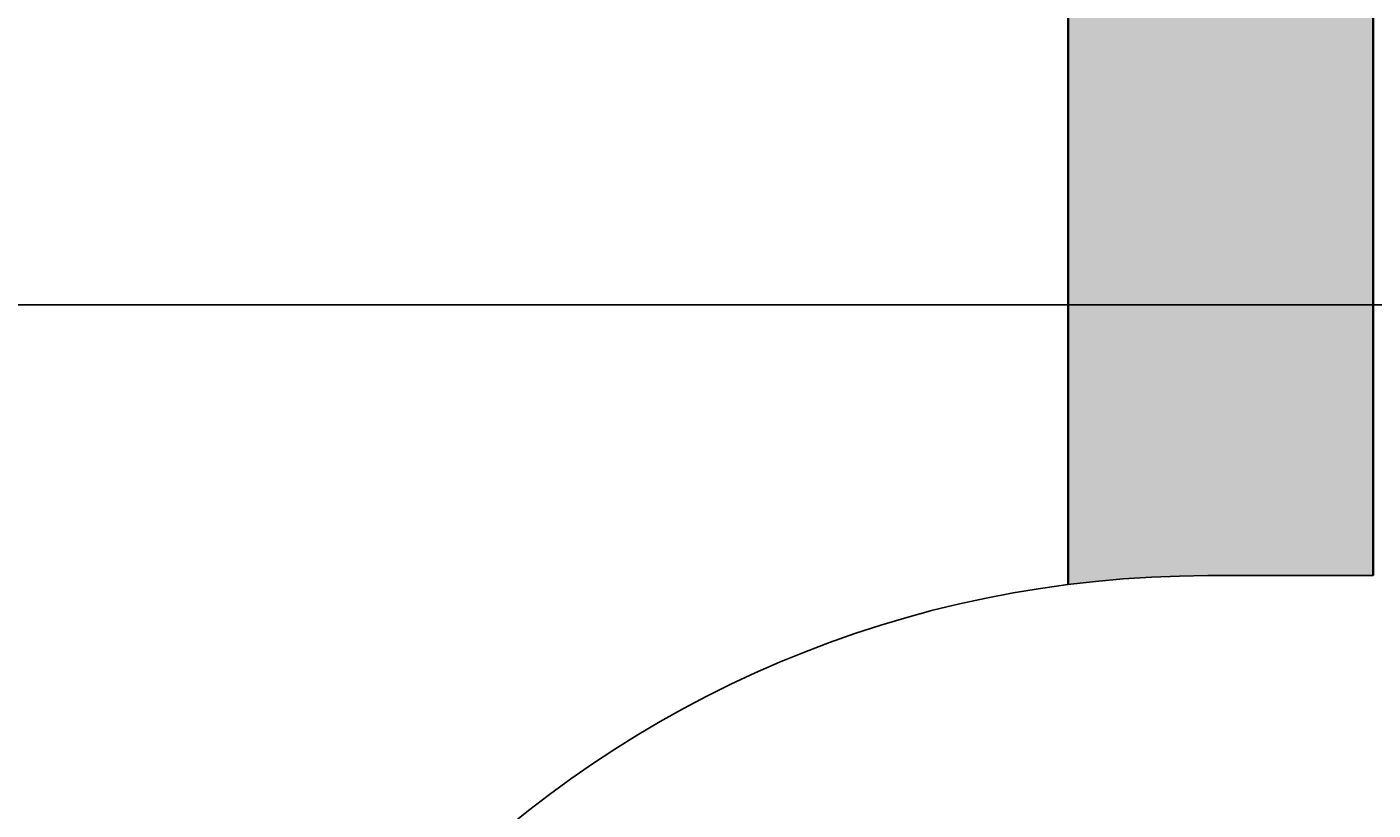
# Model space of a CAD drawing. Units: inches. Extents: x 1998 to 2588, y 1139 to 1977.
# Tile 12 of 134: x 2075 to 2115, y 1622 to 1645. Entities that reach past the tile are written whole.
import ezdxf

# ---------------------------------------------------------------- set-up
doc = ezdxf.new("R2010")
doc.units = ezdxf.units.IN
for name, color, linetype, lineweight in [('A-ANNO-DIMS', 2, 'Continuous', 18), ('A-WALL-PATT', 252, 'Continuous', 13), ('DOOR', 52, 'Continuous', 25), ('WALL', 200, 'Continuous', 35)]:
    doc.layers.add(name, color=color, linetype=linetype, lineweight=lineweight)
doc.styles.get("Standard").update_dxf_attribs({"font": 'arial.ttf'})
doc.dimstyles.get("Standard").update_dxf_attribs({"dimtxt": 0.18, "dimasz": 0.18, "dimexe": 0.18, "dimexo": 0.0625, "dimgap": 0.09, "dimtad": 0, "dimtih": 1, "dimtoh": 1, "dimdec": 4, "dimzin": 0, "dimdsep": 46, "dimtxsty": 'Standard', "dimcen": 0.09, "dimadec": 0, "dimazin": 0, "dimtfac": 1, "dimtdec": 4, "dimtofl": 0, "dimtmove": 0, "dimatfit": 3, "dimfxl": 1, "dimtolj": 1, "dimtzin": 0, "dimarcsym": 0})

# ---------------------------------------------------------------- blocks, each defined once
blk = doc.blocks.new('*U2')
for p, q in [((0, 0), (0, -6)), ((40, 0), (40, -6))]:
    blk.add_line(p, q)
blk.add_lwpolyline([(0, 0), (0, 40), (1.75, 40), (1.75, 0)], close=True)
blk.add_arc((0, 0), 40, 0, 90)
blk = doc.blocks.new('*D30')
at = {"layer": 'A-ANNO-DIMS', "color": 0, "lineweight": -2, "transparency": 16777216}
for p, q in [((2407.91, 1636.732), (1997.843, 1636.732)), ((1998.023, 1636.552), (1998.023, 1615.913)), ((1998.023, 1594.912), (1998.023, 1615.552)), ((2407.91, 1594.732), (1997.843, 1594.732))]:
    blk.add_line(p, q, dxfattribs=at)
at = {"layer": 'A-ANNO-DIMS', "color": 0, "transparency": 16777216}
for points in [[(1997.993, 1636.552), (1998.053, 1636.552), (1998.023, 1636.732)], [(1997.993, 1594.912), (1998.053, 1594.912), (1998.023, 1594.732)]]:
    blk.add_solid(points, dxfattribs=at)
at = {"layer": 'Defpoints', "color": 0, "transparency": 16777216}
for p in [(1998.023, 1636.732), (2407.973, 1636.732), (2407.973, 1594.732)]:
    blk.add_point(p, dxfattribs=at)
at = {"layer": 'A-ANNO-DIMS', "color": 0, "transparency": 16777216, "insert": (1998.023, 1615.732), "char_height": 0.18, "attachment_point": 5}
blk.add_mtext('\\A1;42', dxfattribs=at)
blk = doc.blocks.new('*D38')
at = {"layer": 'A-ANNO-DIMS', "color": 0, "lineweight": -2, "transparency": 16777216}
for p, q in [((2197.387, 1663.247), (1997.843, 1663.247)), ((1998.023, 1663.067), (1998.023, 1638.171)), ((1998.023, 1612.912), (1998.023, 1637.808)), ((2197.387, 1612.732), (1997.843, 1612.732))]:
    blk.add_line(p, q, dxfattribs=at)
at = {"layer": 'A-ANNO-DIMS', "color": 0, "transparency": 16777216}
for points in [[(1997.993, 1663.067), (1998.053, 1663.067), (1998.023, 1663.247)], [(1997.993, 1612.912), (1998.053, 1612.912), (1998.023, 1612.732)]]:
    blk.add_solid(points, dxfattribs=at)
at = {"layer": 'Defpoints', "color": 0, "transparency": 16777216}
for p in [(1998.023, 1663.247), (2197.45, 1663.247), (2197.45, 1612.732)]:
    blk.add_point(p, dxfattribs=at)
at = {"layer": 'A-ANNO-DIMS', "color": 0, "transparency": 16777216, "insert": (1998.023, 1637.99), "char_height": 0.18, "attachment_point": 5}
blk.add_mtext('\\A1;50.51', dxfattribs=at)
blk = doc.blocks.new('*D40')
at = {"layer": 'A-ANNO-DIMS', "color": 0, "lineweight": -2, "transparency": 16777216}
for p, q in [((2105.973, 1628.541), (2105.973, 1977.362)), ((2106.153, 1977.182), (2110.324, 1977.182)), ((2114.793, 1977.182), (2110.622, 1977.182)), ((2114.973, 1628.804), (2114.973, 1977.362))]:
    blk.add_line(p, q, dxfattribs=at)
at = {"layer": 'A-ANNO-DIMS', "color": 0, "transparency": 16777216}
for points in [[(2106.153, 1977.212), (2106.153, 1977.152), (2105.973, 1977.182)], [(2114.793, 1977.212), (2114.793, 1977.152), (2114.973, 1977.182)]]:
    blk.add_solid(points, dxfattribs=at)
at = {"layer": 'Defpoints', "color": 0, "transparency": 16777216}
for p in [(2114.973, 1977.182), (2114.973, 1628.742), (2105.973, 1628.478)]:
    blk.add_point(p, dxfattribs=at)
at = {"layer": 'A-ANNO-DIMS', "color": 0, "transparency": 16777216, "insert": (2110.473, 1977.182), "char_height": 0.18, "attachment_point": 5}
blk.add_mtext('\\A1;9', dxfattribs=at)

msp = doc.modelspace()

# ---------------------------------------------------------------- hatches: boundary and pattern name
at = {"layer": 'A-WALL-PATT'}
h = msp.add_hatch(color=256, dxfattribs=at)
h.dxf.hatch_style = 1
h.paths.add_polyline_path([(2527.4729, 1362.2324), (2510.9729, 1362.2324), (2510.9729, 1357.7324), (2518.4729, 1357.7324), (2518.4729, 1237.7324), (2503.1458, 1237.7324), (2503.1458, 1228.7324), (2527.4729, 1228.7324)])
h.paths.add_polyline_path([(2490.5682, 1362.2324), (2398.4729, 1362.2324), (2398.4729, 1357.7324), (2490.5682, 1357.7324)])
h.paths.add_polyline_path([(2224.9729, 1264.7324), (2222.9729, 1264.7324), (2222.9729, 1232.4125), (2341.4729, 1232.4125), (2341.4729, 1234.4125), (2224.9729, 1234.4125)])
h.paths.add_polyline_path([(2334.5332, 1273.7324), (2264.7638, 1273.7324), (2264.7638, 1269.5611, -0.043659), (2264.3413, 1264.7324), (2334.5332, 1264.7324)])
h.paths.add_polyline_path([(2236.9551, 1273.7324), (2234.4125, 1273.7324), (2234.4125, 1264.7324), (2236.9551, 1264.7324), (2236.9551, 1269.5611)])
h.paths.add_polyline_path([(2222.9729, 1293.2324), (2096.9729, 1293.2324), (2096.9729, 1345.0966), (2087.9729, 1345.0966), (2087.9729, 1284.2324), (2222.9729, 1284.2324), (2222.9729, 1285.137)])
h.paths.add_polyline_path([(2096.9729, 1458.7927), (2087.9729, 1458.7927), (2087.9729, 1417.7324), (2087.9729, 1413.2324), (2096.9729, 1413.2324), (2096.9729, 1417.7324)])
h.paths.add_polyline_path([(2096.9729, 1413.2324), (2087.9729, 1413.2324), (2087.9729, 1365.5012), (2096.9729, 1365.5012), (2096.9729, 1369.3358)])
h.paths.add_polyline_path([(2186.2943, 1417.7324), (2138.6074, 1417.7324), (2096.9729, 1417.7324), (2096.9729, 1413.2324), (2138.6074, 1413.2324), (2186.2943, 1413.2324)])
h.paths.add_polyline_path([(2181.4729, 1465.7324), (2176.9729, 1465.7324), (2176.9729, 1451.6434), (2181.4729, 1451.6434)])
h.paths.add_polyline_path([(2181.4729, 1422.1664), (2176.9729, 1422.1664), (2176.9729, 1417.7324), (2181.4729, 1417.7324)])
h.paths.add_polyline_path([(2063.9729, 1465.7324), (2087.9729, 1465.7324), (2087.9729, 1470.2324), (2059.4729, 1470.2324), (2059.4729, 1413.2324), (2087.9729, 1413.2324), (2087.9729, 1417.7324), (2063.9729, 1417.7324)])
h.paths.add_polyline_path([(2181.4729, 1755.2324), (2176.9729, 1755.2324), (2176.9729, 1748.6798), (2177.0513, 1748.6798), (2181.4729, 1748.6798)])
h.paths.add_polyline_path([(2227.4729, 1707.2324), (2220.4647, 1707.2324), (2220.4647, 1702.7324), (2222.9729, 1702.7324), (2222.9729, 1604.637), (2227.4729, 1604.637)])
h.paths.add_polyline_path([(2114.9729, 1702.7324), (2105.9729, 1702.7324), (2105.9729, 1628.4781, -0.0318759), (2110.1012, 1628.7416), (2114.9729, 1628.7416)])
h.paths.add_polyline_path([(2345.9729, 1739.3278), (2341.4729, 1739.3278), (2341.4729, 1647.5211), (2345.9729, 1647.5211)])
h.paths.add_polyline_path([(2350.6273, 1641.2324), (2345.9729, 1641.2324), (2345.9729, 1636.7324), (2350.6273, 1636.7324), (2350.6273, 1639.8729)])
h.paths.add_polyline_path([(2501.9729, 1641.2324), (2407.9729, 1641.2324), (2392.5005, 1641.2324), (2392.5005, 1639.8729), (2392.5005, 1636.7324), (2501.9729, 1636.7324)])
h.paths.add_polyline_path([(2510.9729, 1755.2324), (2501.9729, 1755.2324), (2501.9729, 1641.2324), (2510.9729, 1641.2324)])
h.paths.add_polyline_path([(2549.1786, 1641.2324), (2522.3775, 1641.2324), (2522.3775, 1636.7324), (2540.1786, 1636.7324), (2540.1786, 1480.7324), (2522.3775, 1480.7324), (2522.3775, 1476.2324), (2549.1786, 1476.2324)])
h.paths.add_polyline_path([(2498.1786, 1594.7324), (2407.9729, 1594.7324), (2407.9729, 1585.7324), (2416.9729, 1585.7324), (2489.1786, 1585.7324), (2489.1786, 1531.7324), (2416.9729, 1531.7324), (2407.9729, 1531.7324), (2407.9729, 1522.7324), (2498.1786, 1522.7324)])
h.paths.add_polyline_path([(2351.6437, 1480.7324), (2345.9729, 1480.7324), (2345.9729, 1476.2324), (2351.6437, 1476.2324), (2351.6437, 1477.5919)])
h.paths.add_polyline_path([(2501.9729, 1480.7324), (2498.1786, 1480.7324), (2407.9729, 1480.7324), (2393.5168, 1480.7324), (2393.5168, 1477.5919), (2393.5168, 1476.2324), (2501.9729, 1476.2324)])

# ---------------------------------------------------------------- linework, layer by layer
at = {"layer": 'WALL'}
for p, q in [((2105.9729, 1628.4781), (2105.9729, 1702.7324)), ((2114.9729, 1628.7416), (2114.9729, 1702.7324))]:
    msp.add_line(p, q, dxfattribs=at)

# ---------------------------------------------------------------- block references
at = {"layer": 'DOOR', "xscale": 0.8119355758402486, "yscale": 0.8119355758402486, "zscale": 0.8119355758402486, "rotation": 90.00000000000003}
msp.add_blockref('*U2', (2110.1012, 1596.2642), dxfattribs=at)

# ---------------------------------------------------------------- dimensions: what is measured, and where the dimension line sits
at = {"layer": 'A-ANNO-DIMS'}
dim = msp.add_linear_dim(base=(2114.9729, 1977.1824), p1=(2105.9729, 1628.4781), p2=(2114.9729, 1628.7416), dimstyle='Standard', override={"dimdec": 0, "dimlfac": 1, "dimrnd": 0, "dimzin": 0, "dimdsep": 46, "dimlunit": 2}, dxfattribs=at)
dim.commit()
dim.dimension.update_dxf_attribs({"geometry": '*D40', "text_midpoint": (2110.4729, 1977.1824)})
for base, p1, p2, override, picture, middle in [((1998.0229, 1663.2466), (2197.4499, 1612.7324), (2197.4499, 1663.2466), {"dimdec": 2, "dimlfac": 1, "dimrnd": 0, "dimzin": 0, "dimdsep": 46, "dimlunit": 2}, '*D38', (1998.0229, 1637.9895)), ((1998.0229, 1636.7324), (2407.9729, 1594.7324), (2407.9729, 1636.7324), {"dimdec": 0, "dimlfac": 1, "dimrnd": 0, "dimzin": 0, "dimdsep": 46, "dimlunit": 2}, '*D30', (1998.0229, 1615.7324))]:
    dim = msp.add_linear_dim(base=base, p1=p1, p2=p2, angle=90, dimstyle='Standard', override=override, dxfattribs=at)
    dim.commit()
    dim.dimension.update_dxf_attribs({"geometry": picture, "text_midpoint": middle})

doc.saveas('drawing.dxf')
